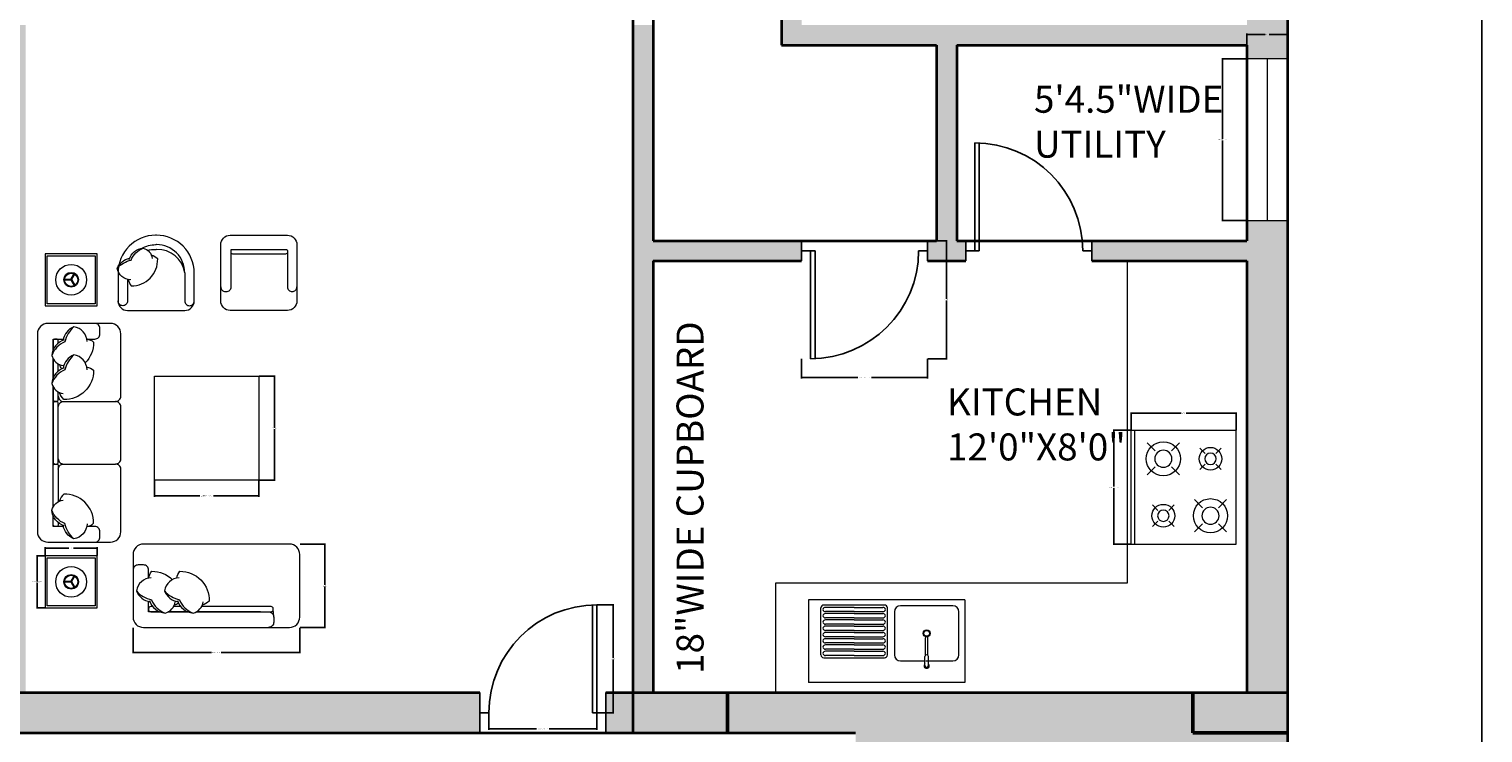
# Model space of a CAD drawing. Units: inches. Extents: x -28 to 485, y -861 to 54.
# Tile 11 of 14: x 162 to 485, y -365 to -208. Entities that reach past the tile are written whole.
import ezdxf

# ---------------------------------------------------------------- set-up
doc = ezdxf.new("R2010")
doc.units = ezdxf.units.IN
doc.header["$MEASUREMENT"] = 0
for name, color, linetype, lineweight in [('A-ANNO-DIMS', 2, 'Continuous', 18), ('A-ANNO-TEXT', 7, 'Continuous', 18), ('A-AREA-IDEN', 7, 'Continuous', 18), ('A-COLS', 7, 'Continuous', 50), ('A-COLS-PATT', 8, 'Continuous', 13), ('A-DOOR', 3, 'Continuous', 25), ('A-EQPM', 9, 'Continuous', 18), ('A-FLOR-CASE', 8, 'Continuous', 18), ('A-FLOR-FIXT', 9, 'Continuous', 18), ('A-FURN', 8, 'Continuous', 13), ('A-GLAZ', 4, 'Continuous', 18), ('A-WALL', 7, 'Continuous', 35), ('A-WALL-PATT', 34, 'Continuous', 13)]:
    doc.layers.add(name, color=color, linetype=linetype, lineweight=lineweight)
doc.styles.get("Standard").update_dxf_attribs({"font": 'arial.ttf'})
doc.dimstyles.get("Standard").update_dxf_attribs({"dimtxt": 0.18, "dimasz": 0.18, "dimexe": 0.18, "dimexo": 0.0625, "dimgap": 0.09, "dimtad": 0, "dimtih": 1, "dimtoh": 1, "dimdec": 0, "dimzin": 0, "dimdsep": 46, "dimlunit": 3, "dimtxsty": 'Standard', "dimcen": 0.09, "dimadec": 0, "dimazin": 0, "dimtfac": 1, "dimtdec": 0, "dimtofl": 0, "dimtmove": 0, "dimatfit": 3, "dimfxl": 1, "dimtolj": 1, "dimtzin": 0, "dimarcsym": 0})

# ---------------------------------------------------------------- blocks, each defined once
blk = doc.blocks.new('DAY BED1')
at = {"color": 0}
blk.add_line((0.3, 0.25), (0.225, 0.255), dxfattribs=at)
blk.add_lwpolyline([(-0.3, 0, -0.414214), (-0.4, 0.1), (-0.4, 0.1, 0.317837), (-0.4, 0.1, -0.414214), (-0.4, 0.1), (-0.4, 0.1, 1.186185), (-0.4, 0.1, -0.414214), (-0.4, 0.1), (-0.4, 1.5, -0.414214), (-0.3, 1.6), (0.3, 1.6, -0.414214), (0.4, 1.5), (0.4, 0.1, -0.414214), (0.3, 0)], format="xyb", close=True, dxfattribs=at)
for points in [[(-0.073, 1.45), (-0.15, 1.45, -0.414214), (-0.2, 1.5), (-0.2, 1.55, -0.414214), (-0.15, 1.6)], [(-0.076, 1.425, -0.356772), (0.05, 1.568, -0.249542), (0.154, 1.438, 9.61688)], [(0.05, 1.568, -0.14773), (0.136, 1.422, -0.213343), (0.262, 1.293, -0.178662)], [(-0.073, 1.45, 0.165541), (-0.139, 1.419, 0.200231), (-0.058, 1.221, 0.121523)], [(0.143, 1.442, -0.306663), (0.262, 1.293, -0.30633), (0.154, 1.196, 0.872847)], [(0.25, 1.345), (0.25, 1.45), (0.152, 1.45, -0.414214)], [(0.2, 1.412), (0.2, 1.43, -0.414214), (0.22, 1.45), (0.23, 1.45, -0.414214), (0.25, 1.43)], [(0.25, 1.43), (0.25, 1.345, -0.414214)], [(-0.076, 1.156, -0.356772), (0.05, 1.299, -0.249542), (0.154, 1.169, 9.61688)], [(0.05, 1.299, -0.14773), (0.136, 1.153, -0.213343), (0.262, 1.024, -0.178662)], [(0.25, 1.262), (0.25, 1.075, -0.414214)], [(-0.073, 1.181, 0.165541), (-0.139, 1.15, 0.425989), (0.148, 0.869, 0.121523), (0.187, 0.936, -7.115464)], [(0.143, 1.173, -0.306663), (0.262, 1.024, -0.30633), (0.154, 0.926, 0.872847)], [(0.168, 1.163, 0.071865), (0.187, 1.205, -7.115464)], [(0.2, 1.142), (0.2, 1.211, -0.414214)], [(0.25, 0.992), (0.25, 0.275, -0.414214), (0.23, 0.255), (0.22, 0.255, -0.414214), (0.2, 0.275), (0.2, 0.942, -0.414214)], [(0.25, 0.377), (0.25, 0.3, 0.414214), (0.3, 0.25), (0.35, 0.25, 0.414214), (0.4, 0.3)]]:
    blk.add_lwpolyline(points, format="xyb", dxfattribs=at)
for points in [[(0.25, 1.075), (0.25, 1.262)], [(0.25, 0.377), (0.25, 0.992)]]:
    blk.add_lwpolyline(points, dxfattribs=at)
blk = doc.blocks.new('COOKTOP-FOUR-BURNER')
for p, q in [((0, 0), (0, 25.33)), ((0, 25.33), (23.39, 25.33)), ((0.84, 0), (0.84, 25.33)), ((23.39, 0), (23.39, 25.33)), ((5.39, 20.79), (3.59, 22.58)), ((8.97, 20.79), (10.76, 22.58)), ((16.47, 20.19), (15.27, 21.39)), ((18.85, 20.19), (20.05, 21.39)), ((5.39, 17.21), (3.59, 15.42)), ((8.97, 17.21), (10.76, 15.42)), ((16.47, 17.8), (15.27, 16.61)), ((18.85, 17.8), (20.05, 16.61)), ((15.87, 8.12), (14.08, 9.91)), ((19.45, 8.12), (21.24, 9.91)), ((5.98, 7.53), (4.79, 8.72)), ((8.37, 7.53), (9.57, 8.72)), ((5.98, 5.14), (4.79, 3.94)), ((8.37, 5.14), (9.57, 3.94)), ((15.87, 4.54), (14.08, 2.75)), ((19.45, 4.54), (21.24, 2.75)), ((0, 0), (23.39, 0))]:
    blk.add_line(p, q)
for centre, radius in [((7.18, 19), 3.8), ((17.66, 19), 2.53), ((17.66, 6.33), 3.8), ((7.18, 6.33), 2.53)]:
    blk.add_circle(centre, radius)
for centre, radius, start, end in [((7.18, 19), 1.9, 90, 270), ((7.18, 19), 1.9, 270, 90), ((17.66, 19), 1.27, 90, 270), ((17.66, 19), 1.27, 270, 90), ((7.18, 6.33), 1.27, 90, 270), ((7.18, 6.33), 1.27, 270, 90), ((17.66, 6.33), 1.9, 90, 270), ((17.66, 6.33), 1.9, 270, 90)]:
    blk.add_arc(centre, radius, start, end)
blk = doc.blocks.new('TABLE-END-WITH-LAMP')
for p, q in [((5.73, 5.83), (6.55, 7.24)), ((5.86, 5.76), (6.67, 7.17)), ((5.79, 5.87), (4.16, 5.87)), ((5.79, 5.72), (4.16, 5.72)), ((5.73, 5.76), (6.55, 4.34)), ((5.86, 5.83), (6.67, 4.41))]:
    blk.add_line(p, q)
at = {"ltscale": 0.03}
blk.add_lwpolyline([(11.59, 0), (11.59, 11.58), (0, 11.58), (0, 0)], close=True, dxfattribs=at)
blk.add_lwpolyline([(11.12, 11.12), (11.12, 0.46), (0.46, 0.46), (0.46, 11.12)], close=True)
for radius in [3.42, 1.64, 1.47]:
    blk.add_circle((5.79, 5.79), radius)
blk = doc.blocks.new('TABLE-COFFEE-SQUARE')
at = {"ltscale": 0.03}
blk.add_lwpolyline([(23.17, 23.17), (23.17, 0), (0, 0), (0, 23.17)], close=True, dxfattribs=at)
blk = doc.blocks.new('DOOR-SWING-24')
for p, q in [((2, 2.25), (2, 26.25)), ((3, 2.25), (3, 26.25)), ((0, 4.5), (0, 0)), ((28, 2.25), (28, 4.5)), ((0, 2.25), (2, 2.25)), ((2, 2.25), (3, 2.25)), ((26, 2.25), (28, 2.25)), ((28, 2.25), (28, 0))]:
    blk.add_line(p, q)
blk.add_arc((2, 2.25), 24, 0, 90)
blk = doc.blocks.new('DOOR-SWING-KITCHEN')
for p, q in [((0, 24), (0, 26.25)), ((28, 21.75), (28, 26.25)), ((2, 24), (0, 24)), ((0, 24), (0, 21.75)), ((2, 24), (2, 0)), ((3, 24), (2, 24)), ((3, 24), (3, 0)), ((28, 24), (26, 24))]:
    blk.add_line(p, q)
blk.add_arc((2, 24), 24, 270, 0)
blk = doc.blocks.new('DOOR-ENTRY-LEAF')
for p, q in [((23, 0), (23, 24)), ((24, 24), (24, 0)), ((23, 0), (24, 0))]:
    blk.add_line(p, q)
blk.add_arc((24, 0), 24, 90, 180)
blk = doc.blocks.new('WINDOW-36IN')
for p, q in [((0, 36), (0, 0)), ((9, 36), (0, 36)), ((4.5, 36), (4.5, 0)), ((9, 0), (9, 36)), ((0, 0), (9, 0))]:
    blk.add_line(p, q)
blk = doc.blocks.new('*D32')
at = {"layer": 'A-ANNO-DIMS', "color": 0, "lineweight": -2, "transparency": 16777216}
for p, q in [((165.06, -325.47), (163.21, -325.47)), ((163.39, -325.65), (163.39, -331.08)), ((163.39, -336.87), (163.39, -331.44)), ((165.06, -337.05), (163.21, -337.05))]:
    blk.add_line(p, q, dxfattribs=at)
at = {"layer": 'A-ANNO-DIMS', "color": 0, "transparency": 16777216}
for points in [[(163.36, -325.65), (163.42, -325.65), (163.39, -325.47)], [(163.36, -336.87), (163.42, -336.87), (163.39, -337.05)]]:
    blk.add_solid(points, dxfattribs=at)
at = {"layer": 'Defpoints', "color": 0, "transparency": 16777216}
for p in [(163.39, -325.47), (165.12, -325.47), (165.12, -337.05)]:
    blk.add_point(p, dxfattribs=at)
at = {"layer": 'A-ANNO-DIMS', "color": 0, "transparency": 16777216, "insert": (163.39, -331.26), "char_height": 0.18, "attachment_point": 5}
blk.add_mtext('\\A1;END TABLE 12 TYP.', dxfattribs=at)
blk = doc.blocks.new('*D33')
at = {"layer": 'A-ANNO-DIMS', "color": 0, "lineweight": -2, "transparency": 16777216}
for p, q in [((165.12, -325.4), (165.12, -323.55)), ((165.3, -323.73), (170.4, -323.73)), ((176.53, -323.73), (171.44, -323.73)), ((176.71, -325.4), (176.71, -323.55))]:
    blk.add_line(p, q, dxfattribs=at)
at = {"layer": 'A-ANNO-DIMS', "color": 0, "transparency": 16777216}
for points in [[(165.3, -323.7), (165.3, -323.76), (165.12, -323.73)], [(176.53, -323.7), (176.53, -323.76), (176.71, -323.73)]]:
    blk.add_solid(points, dxfattribs=at)
at = {"layer": 'Defpoints', "color": 0, "transparency": 16777216}
for p in [(165.12, -325.47), (176.71, -323.73), (176.71, -325.47)]:
    blk.add_point(p, dxfattribs=at)
at = {"layer": 'A-ANNO-DIMS', "color": 0, "transparency": 16777216, "insert": (170.92, -323.73), "char_height": 0.18, "attachment_point": 5}
blk.add_mtext('\\A1;12 TYP.', dxfattribs=at)
blk = doc.blocks.new('*D38')
at = {"layer": 'A-ANNO-DIMS', "color": 0, "lineweight": -2, "transparency": 16777216}
for p, q in [((184.66, -341.46), (184.66, -347.14)), ((221.73, -341.46), (221.73, -347.14)), ((184.84, -346.96), (202.12, -346.96)), ((221.55, -346.96), (204.27, -346.96))]:
    blk.add_line(p, q, dxfattribs=at)
at = {"layer": 'A-ANNO-DIMS', "color": 0, "transparency": 16777216}
for points in [[(184.84, -346.93), (184.84, -346.99), (184.66, -346.96)], [(221.55, -346.93), (221.55, -346.99), (221.73, -346.96)]]:
    blk.add_solid(points, dxfattribs=at)
at = {"layer": 'Defpoints', "color": 0, "transparency": 16777216}
for p in [(184.66, -341.4), (221.73, -341.4), (184.66, -346.96)]:
    blk.add_point(p, dxfattribs=at)
at = {"layer": 'A-ANNO-DIMS', "color": 0, "transparency": 16777216, "insert": (203.2, -346.96), "char_height": 0.18, "attachment_point": 5}
blk.add_mtext('\\A1;DAYBED 37 TYP.', dxfattribs=at)
blk = doc.blocks.new('*D39')
at = {"layer": 'A-ANNO-DIMS', "color": 0, "lineweight": -2, "transparency": 16777216}
for p, q in [((221.8, -322.86), (227.48, -322.86)), ((227.3, -323.04), (227.3, -331.95)), ((227.3, -341.22), (227.3, -332.31)), ((221.8, -341.4), (227.48, -341.4))]:
    blk.add_line(p, q, dxfattribs=at)
at = {"layer": 'A-ANNO-DIMS', "color": 0, "transparency": 16777216}
for points in [[(227.27, -323.04), (227.33, -323.04), (227.3, -322.86)], [(227.27, -341.22), (227.33, -341.22), (227.3, -341.4)]]:
    blk.add_solid(points, dxfattribs=at)
at = {"layer": 'Defpoints', "color": 0, "transparency": 16777216}
for p in [(221.73, -322.86), (221.73, -341.4), (227.3, -341.4)]:
    blk.add_point(p, dxfattribs=at)
at = {"layer": 'A-ANNO-DIMS', "color": 0, "transparency": 16777216, "insert": (227.3, -332.13), "char_height": 0.18, "attachment_point": 5}
blk.add_mtext('\\A1;19 TYP.', dxfattribs=at)
blk = doc.blocks.new('*D40')
at = {"layer": 'A-ANNO-DIMS', "color": 0, "lineweight": -2, "transparency": 16777216}
for p, q in [((406.46, -297.55), (402.54, -297.55)), ((402.72, -297.73), (402.72, -310.03)), ((402.72, -322.7), (402.72, -310.4)), ((406.46, -322.88), (402.54, -322.88))]:
    blk.add_line(p, q, dxfattribs=at)
at = {"layer": 'A-ANNO-DIMS', "color": 0, "transparency": 16777216}
for points in [[(402.69, -297.73), (402.75, -297.73), (402.72, -297.55)], [(402.69, -322.7), (402.75, -322.7), (402.72, -322.88)]]:
    blk.add_solid(points, dxfattribs=at)
at = {"layer": 'Defpoints', "color": 0, "transparency": 16777216}
for p in [(402.72, -297.55), (406.52, -297.55), (406.52, -322.88)]:
    blk.add_point(p, dxfattribs=at)
at = {"layer": 'A-ANNO-DIMS', "color": 0, "transparency": 16777216, "insert": (402.72, -310.22), "char_height": 0.18, "attachment_point": 5}
blk.add_mtext('\\A1;COOKTOP 25 TYP.', dxfattribs=at)
blk = doc.blocks.new('*D41')
at = {"layer": 'A-ANNO-DIMS', "color": 0, "lineweight": -2, "transparency": 16777216}
for p, q in [((406.52, -297.49), (406.52, -293.57)), ((406.7, -293.75), (417.68, -293.75)), ((429.73, -293.75), (418.74, -293.75)), ((429.91, -297.49), (429.91, -293.57))]:
    blk.add_line(p, q, dxfattribs=at)
at = {"layer": 'A-ANNO-DIMS', "color": 0, "transparency": 16777216}
for points in [[(406.7, -293.72), (406.7, -293.78), (406.52, -293.75)], [(429.73, -293.72), (429.73, -293.78), (429.91, -293.75)]]:
    blk.add_solid(points, dxfattribs=at)
at = {"layer": 'Defpoints', "color": 0, "transparency": 16777216}
for p in [(429.91, -293.75), (406.52, -297.55), (429.91, -297.55)]:
    blk.add_point(p, dxfattribs=at)
at = {"layer": 'A-ANNO-DIMS', "color": 0, "transparency": 16777216, "insert": (418.21, -293.75), "char_height": 0.18, "attachment_point": 5}
blk.add_mtext('\\A1;23 TYP.', dxfattribs=at)
blk = doc.blocks.new('*D44')
at = {"layer": 'A-ANNO-DIMS', "color": 0, "lineweight": -2, "transparency": 16777216}
for p, q in [((189.45, -308.73), (189.45, -312.32)), ((212.62, -308.73), (212.62, -312.32)), ((189.63, -312.14), (199.53, -312.14)), ((212.44, -312.14), (202.54, -312.14))]:
    blk.add_line(p, q, dxfattribs=at)
at = {"layer": 'A-ANNO-DIMS', "color": 0, "transparency": 16777216}
for points in [[(189.63, -312.11), (189.63, -312.17), (189.45, -312.14)], [(212.44, -312.11), (212.44, -312.17), (212.62, -312.14)]]:
    blk.add_solid(points, dxfattribs=at)
at = {"layer": 'Defpoints', "color": 0, "transparency": 16777216}
for p in [(189.45, -308.67), (212.62, -308.67), (212.62, -312.14)]:
    blk.add_point(p, dxfattribs=at)
at = {"layer": 'A-ANNO-DIMS', "color": 0, "transparency": 16777216, "insert": (201.04, -312.14), "char_height": 0.18, "attachment_point": 5}
blk.add_mtext('\\A1;COFFEE TABLE 23 TYP.', dxfattribs=at)
blk = doc.blocks.new('*D45')
at = {"layer": 'A-ANNO-DIMS', "color": 0, "lineweight": -2, "transparency": 16777216}
for p, q in [((212.68, -285.5), (216.28, -285.5)), ((216.1, -285.68), (216.1, -296.9)), ((216.1, -308.49), (216.1, -297.26)), ((212.68, -308.67), (216.28, -308.67))]:
    blk.add_line(p, q, dxfattribs=at)
at = {"layer": 'A-ANNO-DIMS', "color": 0, "transparency": 16777216}
for points in [[(216.07, -285.68), (216.13, -285.68), (216.1, -285.5)], [(216.07, -308.49), (216.13, -308.49), (216.1, -308.67)]]:
    blk.add_solid(points, dxfattribs=at)
at = {"layer": 'Defpoints', "color": 0, "transparency": 16777216}
for p in [(212.62, -285.5), (216.1, -285.5), (212.62, -308.67)]:
    blk.add_point(p, dxfattribs=at)
at = {"layer": 'A-ANNO-DIMS', "color": 0, "transparency": 16777216, "insert": (216.1, -297.08), "char_height": 0.18, "attachment_point": 5}
blk.add_mtext('\\A1;23 TYP.', dxfattribs=at)
blk = doc.blocks.new('*D46')
at = {"layer": 'A-ANNO-DIMS', "color": 0, "lineweight": -2, "transparency": 16777216}
for p, q in [((333.28, -281.68), (333.28, -286)), ((361.28, -281.68), (361.28, -286)), ((333.46, -285.82), (345.76, -285.82)), ((361.1, -285.82), (348.81, -285.82))]:
    blk.add_line(p, q, dxfattribs=at)
at = {"layer": 'A-ANNO-DIMS', "color": 0, "transparency": 16777216}
for points in [[(333.46, -285.79), (333.46, -285.85), (333.28, -285.82)], [(361.1, -285.79), (361.1, -285.85), (361.28, -285.82)]]:
    blk.add_solid(points, dxfattribs=at)
at = {"layer": 'Defpoints', "color": 0, "transparency": 16777216}
for p in [(333.28, -281.62), (361.28, -281.62), (361.28, -285.82)]:
    blk.add_point(p, dxfattribs=at)
at = {"layer": 'A-ANNO-DIMS', "color": 0, "transparency": 16777216, "insert": (347.28, -285.82), "char_height": 0.18, "attachment_point": 5}
blk.add_mtext('\\A1;KITCHEN DOOR 28 TYP.', dxfattribs=at)
blk = doc.blocks.new('*D47')
at = {"layer": 'A-ANNO-DIMS', "color": 0, "lineweight": -2, "transparency": 16777216}
for p, q in [((361.35, -255.37), (365.66, -255.37)), ((365.48, -255.55), (365.48, -268.31)), ((365.48, -281.44), (365.48, -268.67)), ((361.35, -281.62), (365.66, -281.62))]:
    blk.add_line(p, q, dxfattribs=at)
at = {"layer": 'A-ANNO-DIMS', "color": 0, "transparency": 16777216}
for points in [[(365.45, -255.55), (365.51, -255.55), (365.48, -255.37)], [(365.45, -281.44), (365.51, -281.44), (365.48, -281.62)]]:
    blk.add_solid(points, dxfattribs=at)
at = {"layer": 'Defpoints', "color": 0, "transparency": 16777216}
for p in [(361.28, -255.37), (365.48, -255.37), (361.28, -281.62)]:
    blk.add_point(p, dxfattribs=at)
at = {"layer": 'A-ANNO-DIMS', "color": 0, "transparency": 16777216, "insert": (365.48, -268.49), "char_height": 0.18, "attachment_point": 5}
blk.add_mtext('\\A1;26 TYP.', dxfattribs=at)
blk = doc.blocks.new('*D48')
at = {"layer": 'A-ANNO-DIMS', "color": 0, "lineweight": -2, "transparency": 16777216}
for p, q in [((263.78, -360.43), (263.78, -364.15)), ((287.78, -360.43), (287.78, -364.15)), ((263.96, -363.97), (274.39, -363.97)), ((287.6, -363.97), (277.18, -363.97))]:
    blk.add_line(p, q, dxfattribs=at)
at = {"layer": 'A-ANNO-DIMS', "color": 0, "transparency": 16777216}
for points in [[(263.96, -363.94), (263.96, -364), (263.78, -363.97)], [(287.6, -363.94), (287.6, -364), (287.78, -363.97)]]:
    blk.add_solid(points, dxfattribs=at)
at = {"layer": 'Defpoints', "color": 0, "transparency": 16777216}
for p in [(263.78, -360.37), (287.78, -360.37), (287.78, -363.97)]:
    blk.add_point(p, dxfattribs=at)
at = {"layer": 'A-ANNO-DIMS', "color": 0, "transparency": 16777216, "insert": (275.78, -363.97), "char_height": 0.18, "attachment_point": 5}
blk.add_mtext('\\A1;ENTRY DOOR 24 TYP.', dxfattribs=at)
blk = doc.blocks.new('*D49')
at = {"layer": 'A-ANNO-DIMS', "color": 0, "lineweight": -2, "transparency": 16777216}
for p, q in [((287.85, -336.37), (291.56, -336.37)), ((291.38, -336.55), (291.38, -348.19)), ((291.38, -360.19), (291.38, -348.55)), ((287.85, -360.37), (291.56, -360.37))]:
    blk.add_line(p, q, dxfattribs=at)
at = {"layer": 'A-ANNO-DIMS', "color": 0, "transparency": 16777216}
for points in [[(291.35, -336.55), (291.41, -336.55), (291.38, -336.37)], [(291.35, -360.19), (291.41, -360.19), (291.38, -360.37)]]:
    blk.add_solid(points, dxfattribs=at)
at = {"layer": 'Defpoints', "color": 0, "transparency": 16777216}
for p in [(287.78, -336.37), (291.38, -336.37), (287.78, -360.37)]:
    blk.add_point(p, dxfattribs=at)
at = {"layer": 'A-ANNO-DIMS', "color": 0, "transparency": 16777216, "insert": (291.38, -348.37), "char_height": 0.18, "attachment_point": 5}
blk.add_mtext('\\A1;24 TYP.', dxfattribs=at)
blk = doc.blocks.new('*D50')
at = {"layer": 'A-ANNO-DIMS', "color": 0, "lineweight": -2, "transparency": 16777216}
for p, q in [((432.22, -214.89), (426.7, -214.89)), ((426.88, -215.07), (426.88, -232.71)), ((426.88, -250.71), (426.88, -233.08)), ((432.22, -250.89), (426.7, -250.89))]:
    blk.add_line(p, q, dxfattribs=at)
at = {"layer": 'A-ANNO-DIMS', "color": 0, "transparency": 16777216}
for points in [[(426.85, -215.07), (426.91, -215.07), (426.88, -214.89)], [(426.85, -250.71), (426.91, -250.71), (426.88, -250.89)]]:
    blk.add_solid(points, dxfattribs=at)
at = {"layer": 'Defpoints', "color": 0, "transparency": 16777216}
for p in [(426.88, -214.89), (432.28, -214.89), (432.28, -250.89)]:
    blk.add_point(p, dxfattribs=at)
at = {"layer": 'A-ANNO-DIMS', "color": 0, "transparency": 16777216, "insert": (426.88, -232.89), "char_height": 0.18, "attachment_point": 5}
blk.add_mtext('\\A1;WINDOW 36 TYP.', dxfattribs=at)
blk = doc.blocks.new('*D51')
at = {"layer": 'A-ANNO-DIMS', "color": 0, "lineweight": -2, "transparency": 16777216}
for p, q in [((432.28, -214.83), (432.28, -209.31)), ((432.46, -209.49), (436.33, -209.49)), ((441.1, -209.49), (437.24, -209.49)), ((441.28, -214.83), (441.28, -209.31))]:
    blk.add_line(p, q, dxfattribs=at)
at = {"layer": 'A-ANNO-DIMS', "color": 0, "transparency": 16777216}
for points in [[(432.46, -209.46), (432.46, -209.52), (432.28, -209.49)], [(441.1, -209.46), (441.1, -209.52), (441.28, -209.49)]]:
    blk.add_solid(points, dxfattribs=at)
at = {"layer": 'Defpoints', "color": 0, "transparency": 16777216}
for p in [(441.28, -209.49), (432.28, -214.89), (441.28, -214.89)]:
    blk.add_point(p, dxfattribs=at)
at = {"layer": 'A-ANNO-DIMS', "color": 0, "transparency": 16777216, "insert": (436.78, -209.49), "char_height": 0.18, "attachment_point": 5}
blk.add_mtext('\\A1;9 TYP.', dxfattribs=at)
blk = doc.blocks.new('*D53')
at = {"layer": 'A-ANNO-DIMS', "color": 0, "lineweight": -2, "transparency": 16777216}
for p, q in [((441.35, 10.13), (484.71, 10.13)), ((484.53, 9.95), (484.53, -403.68)), ((484.53, -817.69), (484.53, -404.05)), ((441.35, -817.87), (484.71, -817.87))]:
    blk.add_line(p, q, dxfattribs=at)
at = {"layer": 'A-ANNO-DIMS', "color": 0, "transparency": 16777216}
for points in [[(484.5, 9.95), (484.56, 9.95), (484.53, 10.13)], [(484.5, -817.69), (484.56, -817.69), (484.53, -817.87)]]:
    blk.add_solid(points, dxfattribs=at)
at = {"layer": 'Defpoints', "color": 0, "transparency": 16777216}
for p in [(441.28, 10.13), (441.28, -817.87), (484.53, -817.87)]:
    blk.add_point(p, dxfattribs=at)
at = {"layer": 'A-ANNO-DIMS', "color": 0, "transparency": 16777216, "insert": (484.53, -403.87), "char_height": 0.18, "attachment_point": 5}
blk.add_mtext('\\A1;828', dxfattribs=at)

msp = doc.modelspace()

# ---------------------------------------------------------------- hatches: boundary and pattern name
at = {"layer": 'A-COLS-PATT'}
h = msp.add_hatch(color=256, dxfattribs=at)
h.dxf.hatch_style = 1
h.paths.add_polyline_path([(36.285, 10.133), (15.285, 10.133), (15.285, 1.133), (36.285, 1.133)])
h.paths.add_polyline_path([(160.785, 10.133), (139.785, 10.133), (139.785, 1.133), (160.785, 1.133)])
h.paths.add_polyline_path([(316.785, 10.133), (295.785, 10.133), (295.785, 1.133), (316.785, 1.133)])
h.paths.add_polyline_path([(441.285, 10.133), (420.285, 10.133), (420.285, 1.133), (441.285, 1.133)])
h.paths.add_polyline_path([(441.285, -138.367), (432.285, -138.367), (420.285, -138.367), (420.285, -147.367), (441.285, -147.367)])
h.paths.add_polyline_path([(304.785, -130.867), (295.785, -130.867), (295.785, -147.367), (304.785, -147.367), (304.785, -142.867)])
h.paths.add_polyline_path([(160.785, -130.867), (151.785, -130.867), (151.785, -142.867), (151.785, -147.367), (160.785, -147.367)])
h.paths.add_polyline_path([(36.285, -138.367), (24.285, -138.367), (15.285, -138.367), (15.285, -147.367), (36.285, -147.367)])
h.paths.add_polyline_path([(36.285, -355.867), (15.285, -355.867), (15.285, -364.867), (36.285, -364.867)])
h.paths.add_polyline_path([(160.785, -355.867), (139.785, -355.867), (139.785, -364.867), (160.785, -364.867)])
h.paths.add_polyline_path([(316.785, -355.867), (300.285, -355.867), (295.785, -355.867), (295.785, -364.867), (316.785, -364.867)])
h = msp.add_hatch(color=256, dxfattribs=at)
h.dxf.hatch_style = 1
h.paths.add_polyline_path([(441.285, -355.867), (420.285, -355.867), (420.285, -364.867), (441.285, -364.867)])
at = {"layer": 'A-WALL-PATT'}
h = msp.add_hatch(color=256, dxfattribs=at)
h.dxf.hatch_style = 1
h.paths.add_polyline_path([(160.785, -808.867), (160.785, -817.867), (295.785, -817.867), (295.785, -808.867)])
h.paths.add_polyline_path([(316.785, -817.867), (323.776, -817.867), (323.776, -808.867), (316.785, -808.867)])
h.paths.add_polyline_path([(420.285, -817.867), (420.285, -808.867), (383.776, -808.867), (383.776, -817.867)])
h.paths.add_polyline_path([(432.285, -808.867), (441.285, -808.867), (441.285, -702.966), (432.285, -702.966), (432.285, -708.367), (397.785, -708.367), (397.785, -710.617), (397.785, -712.867), (432.285, -712.867)])
h.paths.add_polyline_path([(300.285, -712.867), (329.285, -712.867), (329.285, -710.617), (329.285, -708.367), (295.785, -708.367), (295.785, -808.867), (300.285, -808.867)])
h.paths.add_polyline_path([(160.785, -698.867), (158.535, -698.867), (156.285, -698.867), (156.285, -808.867), (160.785, -808.867)])
h.paths.add_polyline_path([(36.285, -808.867), (36.285, -817.867), (79.721, -817.867), (79.721, -808.867)])
h.paths.add_polyline_path([(15.285, -808.867), (24.285, -808.867), (24.285, -739.09), (15.285, -739.09)])
h.paths.add_polyline_path([(24.285, -640.781), (15.285, -640.781), (15.285, -679.09), (24.285, -679.09), (24.285, -664.867), (89.285, -664.867), (89.285, -662.617), (89.285, -660.367), (24.285, -660.367)])
h.paths.add_polyline_path([(15.285, -616.781), (24.285, -616.781), (24.285, -600.367), (15.285, -600.367)])
h.paths.add_polyline_path([(36.285, -595.867), (36.285, -600.367), (123.285, -600.367), (123.285, -660.367), (117.285, -660.367), (117.285, -664.867), (156.285, -664.867), (156.285, -670.867), (160.785, -670.867), (160.785, -660.367), (127.785, -660.367), (127.785, -600.367), (129.785, -600.367), (129.785, -598.117), (129.785, -595.867)])
h.paths.add_polyline_path([(367.785, -664.867), (363.285, -664.867), (363.285, -708.367), (357.285, -708.367), (357.285, -712.867), (369.785, -712.867), (369.785, -708.367), (367.785, -708.367)])
h.paths.add_polyline_path([(432.285, -664.867), (432.285, -666.966), (441.285, -666.966), (441.285, -642.367), (432.285, -642.367), (432.285, -660.367), (328.785, -660.367), (328.785, -664.867), (363.285, -664.867)])
h.paths.add_polyline_path([(333.285, -600.367), (420.285, -600.367), (420.285, -595.867), (326.785, -595.867), (326.785, -600.367), (328.785, -600.367), (328.785, -630.367), (331.035, -630.367), (333.285, -630.367)])
h.paths.add_polyline_path([(441.285, -600.367), (432.285, -600.367), (432.285, -618.367), (441.285, -618.367)])
h.paths.add_polyline_path([(432.285, -591.367), (441.285, -591.367), (441.285, -547.793), (432.285, -547.793)])
h.paths.add_polyline_path([(295.785, -588.367), (300.238, -588.367), (300.285, -583.867), (300.285, -451.867), (295.785, -451.867)])
h.paths.add_polyline_path([(420.285, -451.867), (420.285, -442.867), (316.785, -442.867), (316.785, -451.867)])
h.paths.add_polyline_path([(432.285, -487.793), (441.285, -487.793), (441.285, -451.867), (432.285, -451.867)])
h.paths.add_polyline_path([(432.285, -442.867), (441.285, -442.867), (441.285, -364.867), (432.285, -364.867)])
h.paths.add_polyline_path([(261.785, -451.867), (261.785, -447.367), (261.785, -444.758), (261.785, -442.867), (160.785, -442.867), (160.785, -451.867)])
h.paths.add_polyline_path([(139.785, -451.867), (139.785, -442.867), (36.285, -442.867), (36.285, -451.867)])
h.paths.add_polyline_path([(15.285, -491.617), (24.285, -491.617), (24.285, -451.867), (15.285, -451.867)])
h.paths.add_polyline_path([(24.285, -551.617), (15.285, -551.617), (15.285, -591.367), (24.285, -591.367)])
h.paths.add_polyline_path([(160.785, -451.867), (156.285, -451.867), (156.285, -588.367), (160.785, -588.367)])
h.paths.add_polyline_path([(139.785, -364.867), (139.785, -355.867), (36.285, -355.867), (36.285, -364.867)])
h.paths.add_polyline_path([(24.285, -364.867), (15.285, -364.867), (15.285, -373.867), (24.285, -373.867)])
h.paths.add_polyline_path([(15.285, -433.867), (15.285, -442.867), (24.285, -442.867), (24.285, -433.867)])
h.paths.add_polyline_path([(261.785, -364.867), (261.785, -360.367), (261.785, -355.867), (160.785, -355.867), (160.785, -364.867)])
h.paths.add_polyline_path([(295.785, -355.867), (289.785, -355.867), (289.785, -364.867), (295.785, -364.867)])
h.paths.add_polyline_path([(295.785, -355.867), (300.285, -355.867), (300.285, -259.867), (333.285, -259.867), (333.285, -257.617), (333.285, -255.367), (300.285, -255.367), (300.285, -207.367), (295.785, -207.367)])
h.paths.add_polyline_path([(420.285, -364.867), (420.285, -355.867), (316.785, -355.867), (316.785, -364.867)])
h.paths.add_polyline_path([(24.285, -311.192), (15.285, -311.192), (15.285, -355.867), (24.285, -355.867)])
h.paths.add_polyline_path([(24.285, -211.867), (54.144, -211.867), (54.144, -207.367), (24.285, -207.367), (24.285, -187.772), (15.285, -187.772), (15.285, -251.192), (24.285, -251.192)])
h.paths.add_polyline_path([(82.144, -207.367), (82.144, -209.617), (82.144, -211.867), (127.785, -211.867), (127.785, -147.367), (129.785, -147.367), (129.785, -145.117), (129.785, -142.867), (36.285, -142.867), (36.285, -147.367), (123.285, -147.367), (123.285, -207.367)])
h.paths.add_polyline_path([(160.785, -207.367), (156.285, -207.367), (156.285, -355.867), (160.785, -355.867)])
h.paths.add_polyline_path([(24.285, 1.133), (15.285, 1.133), (15.285, -54.408), (24.285, -54.408)])
h.paths.add_polyline_path([(36.285, 10.133), (36.285, 1.133), (70.235, 1.133), (70.235, 10.133)])
h.paths.add_polyline_path([(15.285, -138.367), (24.285, -138.367), (24.285, -114.408), (15.285, -114.408)])
h.paths.add_polyline_path([(24.285, -147.367), (15.285, -147.367), (15.285, -163.772), (24.285, -163.772)])
h.paths.add_polyline_path([(156.285, -130.867), (160.785, -130.867), (160.785, 1.133), (156.285, 1.133)])
h.paths.add_polyline_path([(130.235, 1.133), (139.785, 1.133), (139.785, 10.133), (130.235, 10.133)])
h.paths.add_polyline_path([(316.785, 10.133), (316.785, 1.133), (328.097, 1.133), (328.097, 10.133)])
h.paths.add_polyline_path([(300.285, 1.133), (295.785, 1.133), (295.785, -130.867), (300.285, -130.867)])
h.paths.add_polyline_path([(420.285, -147.367), (420.285, -142.867), (326.785, -142.867), (326.785, -145.117), (326.785, -147.367), (328.785, -147.367), (328.785, -177.367), (331.035, -177.367), (333.285, -177.367), (333.285, -147.367)])
h.paths.add_polyline_path([(333.285, -207.367), (333.285, -205.367), (328.785, -205.367), (328.785, -211.867), (363.285, -211.867), (363.285, -255.367), (361.285, -255.367), (361.285, -259.867), (369.785, -259.867), (369.785, -255.367), (367.785, -255.367), (367.785, -211.867), (432.285, -211.867), (432.285, -214.893), (441.285, -214.893), (441.285, -188.008), (432.285, -188.008), (432.285, -207.367)])
h.paths.add_polyline_path([(441.285, -250.893), (432.285, -250.893), (432.285, -255.367), (397.785, -255.367), (397.785, -257.617), (397.785, -259.867), (432.285, -259.867), (432.285, -355.867), (441.285, -355.867)])
h.paths.add_polyline_path([(432.285, -138.367), (441.285, -138.367), (441.285, -115.099), (432.285, -115.099)])
h.paths.add_polyline_path([(441.285, -147.367), (432.285, -147.367), (432.285, -164.008), (441.285, -164.008)])
h.paths.add_polyline_path([(420.285, 1.133), (420.285, 10.133), (388.097, 10.133), (388.097, 1.133)])
h.paths.add_polyline_path([(432.285, -55.099), (441.285, -55.099), (441.285, 1.133), (432.285, 1.133)])
h = msp.add_hatch(color=256, dxfattribs=at)
h.dxf.hatch_style = 1
h.paths.add_polyline_path([(441.285, -364.867), (420.285, -364.867), (420.285, -355.867), (316.785, -355.867), (316.785, -364.867), (345.285, -364.867), (345.285, -388.867), (354.285, -388.867), (354.285, -369.367), (432.285, -369.367), (432.285, -438.367), (354.285, -438.367), (354.285, -418.867), (345.285, -418.867), (345.285, -442.867), (316.785, -442.867), (316.785, -451.867), (420.285, -451.867), (420.285, -442.867), (441.285, -442.867)])
h = msp.add_hatch(color=256, dxfattribs=at)
h.dxf.hatch_style = 1
h.paths.add_polyline_path([(354.285, -364.867), (345.285, -364.867), (345.285, -388.867), (354.285, -388.867)])
h.paths.add_polyline_path([(354.285, -418.867), (345.285, -418.867), (345.285, -442.867), (354.285, -442.867)])
h.paths.add_polyline_path([(295.785, -442.867), (289.785, -442.867), (289.785, -451.867), (295.785, -451.867)])

# ---------------------------------------------------------------- linework, layer by layer
at = {"layer": 'A-COLS'}
for p, q in [((316.785, -355.867), (316.785, -364.867)), ((420.285, -355.867), (420.285, -364.867)), ((420.285, -364.867), (441.285, -364.867))]:
    msp.add_line(p, q, dxfattribs=at)
at = {"layer": 'A-DOOR'}
for p, q in [((261.785, -360.367), (261.785, -355.867)), ((289.785, -355.867), (289.785, -364.867)), ((263.785, -360.367), (261.785, -360.367)), ((261.785, -360.367), (261.785, -364.867)), ((289.785, -360.367), (287.785, -360.367))]:
    msp.add_line(p, q, dxfattribs=at)
at = {"layer": 'A-FLOR-CASE'}
for p, q in [((405.672, -259.867), (405.672, -331.525)), ((405.672, -331.525), (327.493, -331.525)), ((327.493, -331.525), (327.493, -355.867))]:
    msp.add_line(p, q, dxfattribs=at)
at = {"layer": 'A-FLOR-FIXT'}
for p, q in [((369.598, -335.284), (334.822, -335.284)), ((334.822, -335.284), (334.822, -353.666)), ((369.598, -335.284), (369.598, -353.666)), ((337.581, -347.522), (337.581, -337.058)), ((351.714, -336.425), (338.214, -336.425)), ((344.964, -336.929), (338.595, -336.929)), ((344.964, -337.879), (338.595, -337.879)), ((344.964, -338.324), (338.595, -338.324)), ((344.964, -339.275), (338.595, -339.275)), ((344.964, -336.929), (351.333, -336.929)), ((344.964, -337.879), (351.333, -337.879)), ((344.964, -338.324), (351.333, -338.324)), ((344.964, -339.275), (351.333, -339.275)), ((352.348, -347.522), (352.348, -337.058)), ((353.902, -337.932), (353.902, -347.485)), ((366.898, -336.563), (355.271, -336.563)), ((368.267, -347.485), (368.267, -337.932)), ((344.964, -339.72), (338.595, -339.72)), ((344.964, -340.67), (338.595, -340.67)), ((344.964, -341.116), (338.595, -341.116)), ((344.964, -342.066), (338.595, -342.066)), ((344.964, -342.511), (338.595, -342.511)), ((344.964, -339.72), (351.333, -339.72)), ((344.964, -340.67), (351.333, -340.67)), ((344.964, -341.116), (351.333, -341.116)), ((344.964, -342.066), (351.333, -342.066)), ((344.964, -342.511), (351.333, -342.511)), ((344.964, -343.462), (338.595, -343.462)), ((344.964, -343.907), (338.595, -343.907)), ((344.964, -344.857), (338.595, -344.857)), ((344.964, -345.303), (338.595, -345.303)), ((344.964, -343.462), (351.333, -343.462)), ((344.964, -343.907), (351.333, -343.907)), ((344.964, -344.857), (351.333, -344.857)), ((344.964, -345.303), (351.333, -345.303)), ((338.214, -348.156), (351.714, -348.156)), ((344.964, -346.253), (338.595, -346.253)), ((344.964, -346.698), (338.595, -346.698)), ((344.964, -347.649), (338.595, -347.649)), ((344.964, -346.253), (351.333, -346.253)), ((344.964, -346.698), (351.333, -346.698)), ((344.964, -347.649), (351.333, -347.649)), ((355.271, -348.854), (360.704, -348.854)), ((360.873, -348.854), (366.898, -348.854)), ((369.598, -353.666), (334.822, -353.666))]:
    msp.add_line(p, q, dxfattribs=at)
for points in [[(360.799, -347.596), (360.799, -343.748)], [(361.37, -347.596), (361.37, -343.748)], [(360.704, -349.922), (360.704, -347.833)], [(361.465, -349.922), (361.465, -347.833)]]:
    msp.add_lwpolyline(points, dxfattribs=at)
for radius in [0.792, 0.634]:
    msp.add_circle((361.085, -342.709), radius, dxfattribs=at)
for centre, radius, start, end in [((338.214, -337.058), 0.634, 90, 180), ((338.595, -337.562), 0.634, 90, 165.50967), ((338.595, -337.245), 0.634, 194.49033, 270), ((338.595, -338.958), 0.634, 90, 165.50967), ((338.595, -338.641), 0.634, 194.49033, 270), ((351.333, -337.562), 0.634, 14.49033, 90), ((351.333, -337.245), 0.634, 270, 345.50967), ((351.333, -338.958), 0.634, 14.49033, 90), ((351.333, -338.641), 0.634, 270, 345.50967), ((351.714, -337.058), 0.634, 0, 90), ((355.271, -337.932), 1.369, 90, 180), ((366.898, -337.932), 1.369, 0, 90), ((338.595, -340.354), 0.634, 90, 165.50967), ((338.595, -340.037), 0.634, 194.49033, 270), ((338.595, -341.749), 0.634, 90, 165.50967), ((338.595, -341.432), 0.634, 194.49033, 270), ((338.595, -343.145), 0.634, 90, 165.50967), ((351.333, -340.354), 0.634, 14.49033, 90), ((351.333, -340.037), 0.634, 270, 345.50967), ((351.333, -341.749), 0.634, 14.49033, 90), ((351.333, -341.432), 0.634, 270, 345.50967), ((351.333, -343.145), 0.634, 14.49033, 90), ((338.595, -342.828), 0.634, 194.49033, 270), ((338.595, -344.541), 0.634, 90, 165.50967), ((338.595, -344.224), 0.634, 194.49033, 270), ((338.595, -345.936), 0.634, 90, 165.50967), ((338.595, -345.619), 0.634, 194.49033, 270), ((351.333, -342.828), 0.634, 270, 345.50967), ((351.333, -344.541), 0.634, 14.49033, 90), ((351.333, -344.224), 0.634, 270, 345.50967), ((351.333, -345.936), 0.634, 14.49033, 90), ((351.333, -345.619), 0.634, 270, 345.50967), ((361.085, -343.722), 0.286, 354.94633, 185.05367), ((338.214, -347.522), 0.634, 180, 270), ((338.595, -347.332), 0.634, 90, 165.50967), ((338.595, -347.015), 0.634, 194.49033, 270), ((351.333, -347.332), 0.634, 14.49033, 90), ((351.333, -347.015), 0.634, 270, 345.50967), ((351.714, -347.522), 0.634, 270, 0), ((355.271, -347.485), 1.369, 180, 270), ((361.085, -347.848), 0.381, 2.21976, 177.78024), ((366.898, -347.485), 1.369, 270, 0), ((361.085, -349.922), 0.569, 131.90178, 48.09822), ((361.085, -349.922), 0.38, 180, 0)]:
    msp.add_arc(centre, radius, start, end, dxfattribs=at)
at = {"layer": 'A-FURN', "ltscale": 0.03}
msp.add_lwpolyline([(189.8, -270.875), (196.172, -270.875, 0.4142136), (198.261, -268.786), (198.261, -262.519, 0.4142136), (189.904, -254.163), (189.8, -254.163), (189.696, -254.163, 0.4142136), (181.339, -262.519), (181.339, -268.786, 0.4142136), (183.428, -270.875), (189.8, -270.875)], format="xyb", dxfattribs=at)
for points in [[(218.999, -254.163), (218.999, -254.163, -0.4142136), (221.088, -256.252), (221.088, -268.786, -0.4142136), (218.999, -270.875), (218.999, -270.875), (206.256, -270.875, -0.4142136), (204.167, -268.786), (204.167, -256.252, -0.4142136), (206.256, -254.163)], [(179.637, -322.422, 0.4142136), (181.954, -320.105), (181.954, -306.203, 0.4142136), (180.796, -305.044, 0.4142136), (181.954, -303.886), (181.954, -292.301, 0.4142136), (180.796, -291.142, 0.4142136), (181.954, -289.984), (181.954, -276.082, 0.4142136), (179.637, -273.765), (165.735, -273.765, 0.4142136), (163.418, -276.082), (163.418, -320.105, 0.4142136), (165.735, -322.422)]]:
    msp.add_lwpolyline(points, format="xyb", close=True, dxfattribs=at)
at = {"layer": 'A-FURN'}
for points in [[(181.168, -261.465, -0.1477299), (184.221, -259.669, -0.2133428), (186.915, -257.036, -0.1786618)], [(183.799, -259.526, -0.3066635), (186.915, -257.036, -0.30633), (188.95, -259.31, 0.8728472)], [(186.585, -257.078, -0.1305915), (189.696, -256.252), (189.8, -256.252)], [(187.915, -257.521, -0.0723842), (189.696, -257.296), (189.8, -257.296)], [(196.172, -262.519, 0.4142136), (189.904, -256.252), (189.8, -256.252)], [(196.172, -262.519, 0.3727189), (189.904, -257.296), (189.8, -257.296)], [(211.452, -258.341), (206.882, -258.341, -0.4142136), (206.465, -257.923), (206.465, -257.714, -0.4142136), (206.882, -257.296)], [(206.882, -257.296), (210.4, -257.296, -0.4142136)], [(210.4, -257.296), (218.581, -257.296, -0.4142136), (218.999, -257.714), (218.999, -257.923, -0.4142136), (218.581, -258.341), (211.452, -258.341, -0.4142136)], [(218.999, -257.923), (218.999, -265.653, 0.4142136), (220.044, -266.697), (220.044, -266.697, 0.4142136), (221.088, -265.653)], [(184.161, -264.097, -0.3567724), (181.168, -261.465, -0.2495421), (183.88, -259.295, 9.6168803)], [(183.635, -264.034, 0.1655406), (184.281, -265.414, 0.4259892), (190.147, -259.43, 0.1215233), (188.755, -258.605, -7.1154643)], [(183.428, -263.984), (183.428, -268.786, -0.4142136), (182.384, -269.831), (182.384, -269.831, -0.4142136), (181.339, -268.786)], [(196.172, -262.519), (196.172, -268.786, 0.4142136), (197.216, -269.831), (197.216, -269.831, 0.4142136), (198.261, -268.786)], [(204.167, -265.653, 0.4142136), (205.211, -266.697), (205.42, -266.697, 0.4142136), (206.465, -265.653), (206.465, -264.034)], [(171.517, -274.502, 0.1477299), (169.526, -277.888, 0.2133428), (166.605, -280.876, 0.1786618)], [(174.437, -277.822, 0.3567724), (171.517, -274.502, 0.2495421), (169.11, -277.51, -9.6168803)], [(174.367, -277.24), (176.162, -277.24, 0.4142136), (177.32, -276.082), (177.32, -274.923, 0.4142136), (176.162, -273.765)], [(169.367, -277.42, 0.3066635), (166.605, -280.876, 0.30633), (169.127, -283.133, -0.8728472)], [(166.894, -279.677), (166.894, -277.24), (169.17, -277.24, 0.4142136)], [(168.052, -278.124), (168.052, -277.704, 0.4142136), (167.589, -277.24), (167.357, -277.24, 0.4142136), (166.894, -277.704)], [(166.894, -277.704), (166.894, -279.677, 0.4142136)], [(174.366, -277.238, -0.1655406), (175.897, -277.954, -0.2002311), (174.033, -282.553, -0.1215233)], [(171.517, -280.743, 0.1477299), (169.526, -284.129, 0.2133428), (166.605, -287.116, 0.1786618)], [(174.437, -284.062, 0.3567724), (171.517, -280.743, 0.2495421), (169.11, -283.751, -9.6168803)], [(169.367, -283.661, 0.3066635), (166.605, -287.116, 0.30633), (169.127, -289.374, -0.8728472)], [(166.894, -281.605), (166.894, -285.918, 0.4142136)], [(168.052, -284.365), (168.052, -282.771, 0.4142136)], [(168.798, -283.888, -0.0718654), (168.345, -282.916, 7.1154643)], [(174.366, -283.479, -0.1655406), (175.897, -284.195, -0.4259892), (169.26, -290.702, -0.1215233), (168.345, -289.157, 7.1154643)], [(166.894, -287.846), (166.894, -290.679, 0.4142136), (167.357, -291.142), (167.589, -291.142, 0.4142136), (168.052, -290.679), (168.052, -289.012, 0.4142136)], [(168.052, -289.984, 0.4142136), (169.211, -291.142), (180.796, -291.142, 0.4142136)], [(168.052, -292.301, -0.4142136), (169.211, -291.142)], [(166.894, -314.582), (166.894, -305.508, -0.4142136), (167.357, -305.044), (167.589, -305.044, -0.4142136), (168.052, -305.508), (168.052, -313.415, -0.4142136)], [(168.052, -303.886, 0.4142136), (169.211, -305.044)], [(168.052, -306.203, -0.4142136), (169.211, -305.044), (180.796, -305.044, -0.4142136)], [(169.367, -318.766, -0.3066635), (166.605, -315.311, -0.30633), (169.127, -313.054, 0.8728472)], [(174.366, -318.949, 0.1655406), (175.897, -318.232, 0.4259892), (169.26, -311.726, 0.1215233), (168.345, -313.27, -7.1154643)], [(171.517, -321.684, -0.1477299), (169.526, -318.298, -0.2133428), (166.605, -315.311, -0.1786618)], [(166.894, -318.483), (166.894, -316.509, -0.4142136)], [(168.052, -318.062), (168.052, -318.483, -0.4142136), (167.589, -318.946), (167.357, -318.946, -0.4142136), (166.894, -318.483)], [(174.437, -318.365, -0.3567724), (171.517, -321.684, -0.2495421), (169.11, -318.677, 9.6168803)], [(176.162, -322.422, 0.4142136), (177.32, -321.263), (177.32, -320.105, 0.4142136), (176.162, -318.946), (174.367, -318.946)]]:
    msp.add_lwpolyline(points, format="xyb", dxfattribs=at)
for points in [[(206.465, -264.034), (206.465, -257.296), (210.4, -257.296)], [(210.4, -257.296), (218.895, -257.296)], [(166.894, -285.918), (166.894, -281.605)], [(166.894, -314.582), (166.894, -287.846)], [(169.17, -318.946), (166.894, -318.946), (166.894, -316.509)]]:
    msp.add_lwpolyline(points, dxfattribs=at)
msp.add_lwpolyline([(166.894, -291.606), (166.894, -304.581, 0.4142136), (167.357, -305.044), (167.589, -305.044, 0.4142136), (168.052, -304.581), (168.052, -291.606, 0.4142136), (167.589, -291.142), (167.357, -291.142, 0.4142136)], format="xyb", close=True, dxfattribs=at)
at = {"layer": 'A-WALL'}
for p, q in [((295.785, 10.133), (295.785, -364.867)), ((441.285, 10.133), (441.285, -817.867)), ((300.285, -147.367), (300.285, -255.367)), ((328.785, -205.367), (328.785, -211.867)), ((328.785, -211.867), (363.285, -211.867)), ((363.285, -211.867), (363.285, -255.367)), ((367.785, -211.867), (367.785, -255.367)), ((367.785, -211.867), (432.285, -211.867)), ((432.285, -211.867), (432.285, -255.367)), ((300.285, -255.367), (363.285, -255.367)), ((367.785, -255.367), (432.285, -255.367)), ((300.285, -259.867), (333.285, -259.867)), ((300.285, -259.867), (300.285, -355.867)), ((361.285, -259.867), (369.785, -259.867)), ((397.785, -259.867), (432.285, -259.867)), ((432.285, -259.867), (432.285, -355.867)), ((15.285, -355.867), (261.785, -355.867)), ((289.785, -355.867), (441.285, -355.867)), ((15.285, -364.867), (345.285, -364.867))]:
    msp.add_line(p, q, dxfattribs=at)

# ---------------------------------------------------------------- block references
at = {"layer": 'A-DOOR'}
for name, p in [('DOOR-SWING-24', (369.785, -259.867)), ('DOOR-SWING-KITCHEN', (333.285, -281.617)), ('DOOR-ENTRY-LEAF', (263.785, -360.367))]:
    msp.add_blockref(name, p, dxfattribs=at)
at = {"layer": 'A-EQPM'}
msp.add_blockref('COOKTOP-FOUR-BURNER', (406.519, -322.882), dxfattribs=at)
at = {"layer": 'A-FURN'}
for name, p in [('TABLE-END-WITH-LAMP', (165.124, -269.857)), ('TABLE-COFFEE-SQUARE', (189.453, -308.667)), ('TABLE-END-WITH-LAMP', (165.124, -337.05))]:
    msp.add_blockref(name, p, dxfattribs=at)
at = {"layer": 'A-FURN', "ltscale": 0.03, "xscale": -23.16998213752128, "yscale": 23.16998213752128, "zscale": 23.16998213752128, "rotation": 90}
msp.add_blockref('DAY BED1', (221.735, -332.129), dxfattribs=at)
at = {"layer": 'A-GLAZ'}
msp.add_blockref('WINDOW-36IN', (432.285, -250.893), dxfattribs=at)

# ---------------------------------------------------------------- texts
at = {"layer": 'A-ANNO-TEXT', "insert": (305.48, -351.731), "char_height": 6, "attachment_point": 1, "rotation": 90}
msp.add_mtext('18"WIDE CUPBOARD', dxfattribs=at)
at = {"layer": 'A-AREA-IDEN', "char_height": 6, "attachment_point": 1}
for s, insert in [('5\'4.5"WIDE\\PUTILITY', (384.943, -220.91)), ('KITCHEN\\P12\'0"X8\'0"', (365.616, -288.247))]:
    msp.add_mtext(s, dxfattribs=dict(at, insert=insert))

# ---------------------------------------------------------------- dimensions: what is measured, and where the dimension line sits
at = {"layer": 'A-ANNO-DIMS'}
dim = msp.add_linear_dim(base=(484.535, -817.867), p1=(441.285, 10.133), p2=(441.285, -817.867), angle=90, dimstyle='Standard', override={"dimdec": 0, "dimlfac": 1, "dimrnd": 0, "dimzin": 0, "dimdsep": 46, "dimlunit": 2}, dxfattribs=at)
dim.commit()
dim.dimension.update_dxf_attribs({"geometry": '*D53', "text_midpoint": (484.535, -403.867)})
for base, p1, p2, text, picture, middle in [((441.285, -209.493), (432.285, -214.893), (441.285, -214.893), '<> TYP.', '*D51', (436.785, -209.493)), ((361.285, -285.817), (333.285, -281.617), (361.285, -281.617), 'KITCHEN DOOR <> TYP.', '*D46', (347.285, -285.817)), ((429.907, -293.753), (406.519, -297.552), (429.907, -297.552), '<> TYP.', '*D41', (418.213, -293.753)), ((212.622, -312.143), (189.452, -308.667), (212.622, -308.667), 'COFFEE TABLE <> TYP.', '*D44', (201.037, -312.143)), ((176.709, -323.728), (165.124, -325.465), (176.709, -325.465), '<> TYP.', '*D33', (170.916, -323.728)), ((287.785, -363.967), (263.785, -360.367), (287.785, -360.367), 'ENTRY DOOR <> TYP.', '*D48', (275.785, -363.967))]:
    dim = msp.add_linear_dim(base=base, p1=p1, p2=p2, text=text, dimstyle='Standard', override={"dimdec": 0, "dimlfac": 1, "dimrnd": 0, "dimzin": 0, "dimdsep": 46, "dimlunit": 2}, dxfattribs=at)
    dim.commit()
    dim.dimension.update_dxf_attribs({"geometry": picture, "text_midpoint": middle})
for base, p1, p2, angle, text, picture, middle in [((426.885, -214.893), (432.285, -250.893), (432.285, -214.893), 90, 'WINDOW <> TYP.', '*D50', (426.885, -232.893)), ((365.485, -255.367), (361.285, -281.617), (361.285, -255.367), 90, '<> TYP.', '*D47', (365.485, -268.492)), ((216.098, -285.497), (212.622, -308.667), (212.622, -285.497), 90, '<> TYP.', '*D45', (216.098, -297.082)), ((402.72, -297.552), (406.519, -322.882), (406.519, -297.552), 90, 'COOKTOP <> TYP.', '*D40', (402.72, -310.217)), ((227.296, -341.397), (221.735, -322.861), (221.735, -341.397), 270, '<> TYP.', '*D39', (227.296, -332.129)), ((163.386, -325.465), (165.124, -337.05), (165.124, -325.465), 90, 'END TABLE <> TYP.', '*D32', (163.386, -331.258)), ((291.385, -336.367), (287.785, -360.367), (287.785, -336.367), 90, '<> TYP.', '*D49', (291.385, -348.367)), ((184.663, -346.958), (221.735, -341.397), (184.663, -341.397), 180, 'DAYBED <> TYP.', '*D38', (203.199, -346.958))]:
    dim = msp.add_linear_dim(base=base, p1=p1, p2=p2, angle=angle, text=text, dimstyle='Standard', override={"dimdec": 0, "dimlfac": 1, "dimrnd": 0, "dimzin": 0, "dimdsep": 46, "dimlunit": 2}, dxfattribs=at)
    dim.commit()
    dim.dimension.update_dxf_attribs({"geometry": picture, "text_midpoint": middle})

doc.saveas('drawing.dxf')
